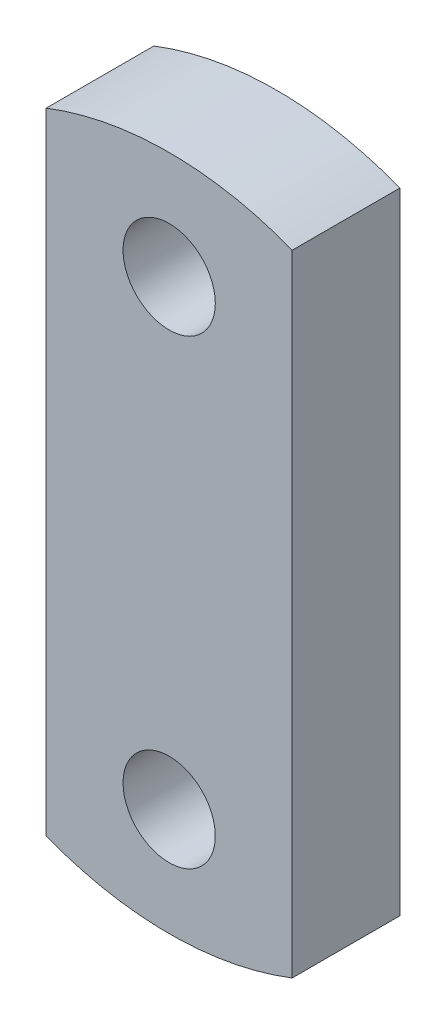
from build123d import *

# Parameters (mm, degrees)
PLATE_PROFILE_WITH_BORES_R = 15
CROSSHEAD_PLATE_35MM_DEPTH = 17.5


with BuildPart() as part:
    # Plate Profile with Bores → Crosshead Plate 35mm (new, symmetric)
    with BuildSketch(Plane.XY):
        with BuildLine():
            Line((-40, -102.46950766), (-40, 102.46950766))
            ThreePointArc((-40, 102.46950766), (0, 110), (40, 102.46950766))
            Line((40, 102.46950766), (40, -102.46950766))
            ThreePointArc((40, -102.46950766), (0, -110), (-40, -102.46950766))
        make_face()
        with Locations((0, 75)):
            Circle(PLATE_PROFILE_WITH_BORES_R, mode=Mode.SUBTRACT)
        with Locations(Location((0, -75, 0), (0, 0, 180))):
            Circle(PLATE_PROFILE_WITH_BORES_R, mode=Mode.SUBTRACT)
    extrude(amount=CROSSHEAD_PLATE_35MM_DEPTH, both=True)


solid = part.part
